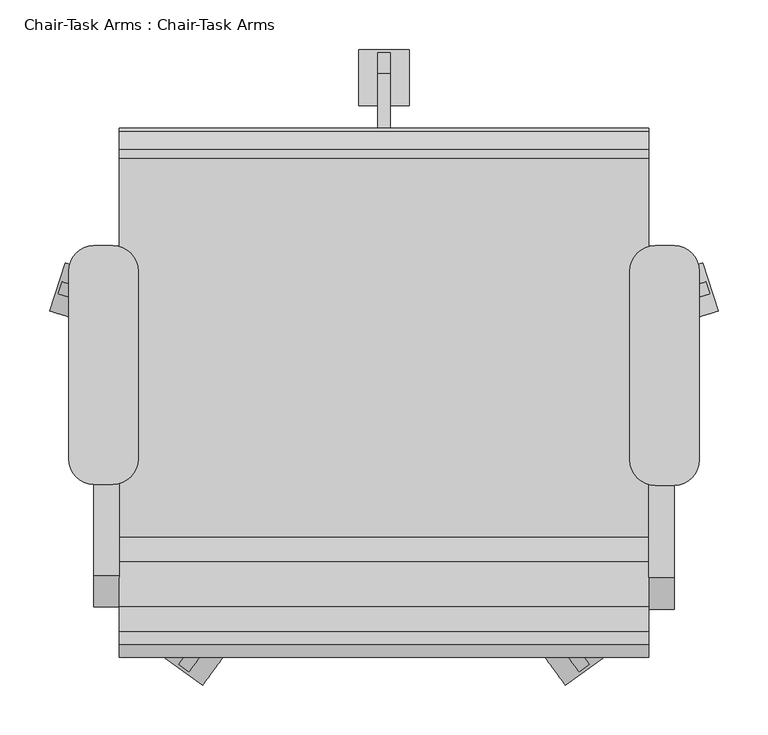
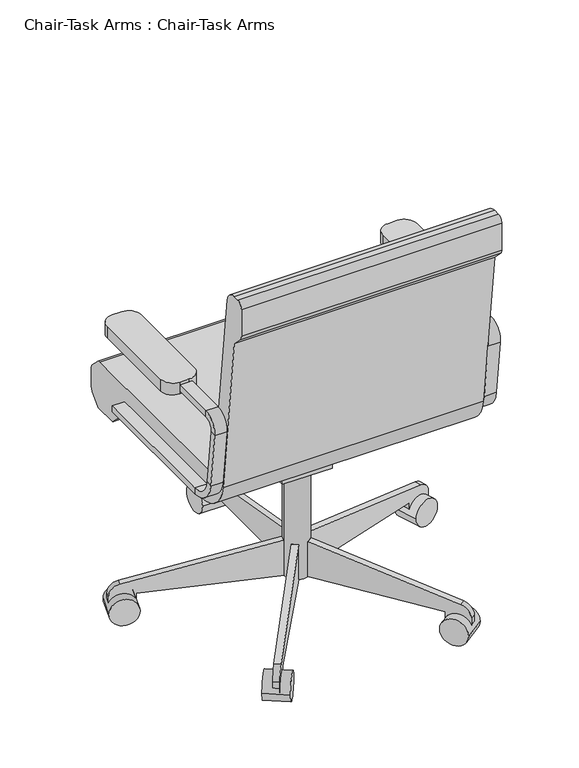
"""IFC4 building model written with IfcOpenShell, lengths in millimetres: furniture geometry, Chair-Task Arms : Chair-Task Arms."""

from ifc_helpers import new_model, si_unit, point, frame, frame_2d, origin, place, context, project, spatial, polyline, circle_curve, trimmed, segment, composite_curve, outline, extrude, source, transform, mapped, element, save
from ifc_brep_helpers import plane_surface, cylinder_surface, revolved_surface, advanced_brep


def chair_task_arms_chair_task_arms_bb362225(model_context):
    return source(origin(), model_context, "Body", "SolidModel", [
        extrude(outline(composite_curve([segment(polyline([(-126.2050455, 457.2), (255.0102301, 457.2)]), True, "CONTINUOUS"), segment(trimmed(circle_curve(frame_2d((255.0102301, 444.5)), 12.7), [point((255.0102301, 457.2))], [point((263.9604301, 453.510212))], False, "CARTESIAN"), True, "CONTINUOUS"), segment(polyline([(263.9604301, 453.510212), (281.8961016, 435.6939999)]), True, "CONTINUOUS"), segment(trimmed(circle_curve(frame_2d((272.9459016, 426.6837879)), 12.7), [point((281.8961016, 435.6939999))], [point((285.6459016, 426.6837879))], False, "CARTESIAN"), True, "CONTINUOUS"), segment(polyline([(285.6459016, 426.6837879), (285.6459016, 391.6405184)]), True, "CONTINUOUS"), segment(trimmed(circle_curve(frame_2d((260.2459016, 391.6405184)), 25.4), [point((285.6459016, 391.6405184))], [point((278.2663256, 373.7401184))], False, "CARTESIAN"), True, "CONTINUOUS"), segment(polyline([(278.2663256, 373.7401184), (260.2470284, 355.6), (209.4470284, 355.6), (181.0744602, 383.7835944), (-107.1089978, 383.7835944)]), True, "CONTINUOUS"), segment(trimmed(circle_curve(frame_2d((-107.1089978, 459.9835944)), 76.2), [point((-107.1089978, 383.7835944))], [point((-182.7870738, 451.0802913))], False, "CARTESIAN"), True, "CONTINUOUS"), segment(polyline([(-182.7870738, 451.0802913), (-222.3540984, 787.4), (-244.0343545, 809.0802561)]), True, "CONTINUOUS"), segment(trimmed(circle_curve(frame_2d((-235.0540984, 818.0605122)), 12.7), [point((-244.0343545, 809.0802561))], [point((-247.7540984, 818.0605122))], False, "CARTESIAN"), True, "CONTINUOUS"), segment(polyline([(-247.7540984, 818.0605122), (-247.7540984, 876.3)]), True, "CONTINUOUS"), segment(trimmed(circle_curve(frame_2d((-235.0540984, 876.3)), 12.7), [point((-247.7540984, 876.3))], [point((-235.0540984, 889.0))], False, "CARTESIAN"), True, "CONTINUOUS"), segment(polyline([(-235.0540984, 889.0), (-222.1789239, 889.0)]), True, "CONTINUOUS"), segment(trimmed(circle_curve(frame_2d((-222.1789239, 863.6)), 25.4), [point((-222.1789239, 889.0))], [point((-196.9528985, 866.5677677))], False, "CARTESIAN"), True, "CONTINUOUS"), segment(polyline([(-196.9528985, 866.5677677), (-151.4310708, 479.6322323)]), True, "CONTINUOUS"), segment(trimmed(circle_curve(frame_2d((-126.2050455, 482.6)), 25.4), [point((-151.4310708, 479.6322323))], [point((-126.2050455, 457.2))], True, "CARTESIAN"), True, "CONTINUOUS")], self_intersect=False)), frame((-125.7091803, 0.0, 0.0), z_axis=(1.0, 0.0, 0.0), x_axis=(0.0, 1.0, 0.0)), (0.0, 0.0, 1.0), 533.4),
        extrude(outline(polyline([(69.7459016, 383.7835944), (69.7459016, 371.0835944), (18.9459016, 283.0954134), (-19.1540984, 283.0954134), (-19.1540984, 383.7835944), (69.7459016, 383.7835944)])), frame((90.1908197, 0.0, 0.0), z_axis=(1.0, 0.0, 0.0), x_axis=(0.0, 1.0, 0.0)), (0.0, 0.0, 1.0), 101.6),
        extrude(outline(composite_curve([segment(polyline([(311.0459016, 53.5835944), (18.9459016, 53.5835944), (18.9459016, 129.7835944), (44.3459016, 129.7835944), (340.8565654, 77.5007643)]), True, "CONTINUOUS"), segment(trimmed(circle_curve(frame_2d((336.4459016, 52.4866474)), 25.4), [point((340.8565654, 77.5007643))], [point((361.8459016, 52.4866474))], False, "CARTESIAN"), True, "CONTINUOUS"), segment(polyline([(361.8459016, 52.4866474), (361.8459016, 28.1835944), (311.0459016, 28.1835944), (311.0459016, 53.5835944)]), True, "CONTINUOUS")], self_intersect=False)), frame((134.6408197, 0.0, 0.0), z_axis=(1.0, 0.0, 0.0), x_axis=(0.0, 1.0, 0.0)), (0.0, 0.0, 1.0), 12.7),
        extrude(outline(composite_curve([segment(trimmed(circle_curve(frame_2d((336.4459016, 28.1835944)), 28.2002727), [point((308.2456289, 28.1835944))], [point((364.6461744, 28.1835944))], False, "CARTESIAN"), True, "CONTINUOUS"), segment(trimmed(circle_curve(frame_2d((336.4459016, 28.1835944)), 28.2002727), [point((364.6461744, 28.1835944))], [point((308.2456289, 28.1835944))], False, "CARTESIAN"), True, "CONTINUOUS")], self_intersect=False)), frame((115.5908197, 0.0, 0.0), z_axis=(1.0, 0.0, 0.0), x_axis=(0.0, 1.0, 0.0)), (0.0, 0.0, 1.0), 50.8),
        extrude(outline(composite_curve([segment(polyline([(25.4, 0.0), (25.4, 292.1000001), (101.6, 292.1000001), (101.6, 266.7), (49.3171699, -29.8106636)]), True, "CONTINUOUS"), segment(trimmed(circle_curve(frame_2d((24.303053, -25.4)), 25.4), [point((49.3171699, -29.8106636))], [point((24.303053, -50.8))], False, "CARTESIAN"), True, "CONTINUOUS"), segment(polyline([(24.303053, -50.8), (0.0, -50.8), (0.0, 0.0), (25.4, 0.0)]), True, "CONTINUOUS")], self_intersect=False)), frame((-138.7750467, 103.1705568, 28.1835944), z_axis=(0.3090169943749487, 0.9510565162951532, 0.0), x_axis=(0.0, 0.0, 1.0)), (0.0, 0.0, 1.0), 12.7),
        extrude(outline(composite_curve([segment(trimmed(circle_curve(frame_2d((0.0, -28.2002727)), 28.2002727), [point((0.0, -56.4005454))], [point((0.0, 0.0))], False, "CARTESIAN"), True, "CONTINUOUS"), segment(trimmed(circle_curve(frame_2d((0.0, -28.2002727)), 28.2002727), [point((0.0, 0.0))], [point((0.0, -56.4005454))], False, "CARTESIAN"), True, "CONTINUOUS")], self_intersect=False)), frame((-195.638709, 101.6163254, 28.1835944), z_axis=(0.3090169943749487, 0.9510565162951532, 0.0), x_axis=(0.0, 0.0, -1.0)), (0.0, 0.0, 1.0), 50.8),
        extrude(outline(composite_curve([segment(polyline([(25.4, 0.0), (25.4, 292.1), (101.6, 292.1), (101.6, 266.7), (49.3171699, -29.8106637)]), True, "CONTINUOUS"), segment(trimmed(circle_curve(frame_2d((24.303053, -25.3999999)), 25.4), [point((49.3171699, -29.8106637))], [point((24.303053, -50.8))], False, "CARTESIAN"), True, "CONTINUOUS"), segment(polyline([(24.303053, -50.8), (0.0, -50.8), (0.0, 0.0), (25.4, 0.0)]), True, "CONTINUOUS")], self_intersect=False)), frame((-25.5639946, -221.1003988, 28.1835944), z_axis=(-0.8090169943749459, 0.5877852522924754, 0.0), x_axis=(0.0, 0.0, 1.0)), (0.0, 0.0, 1.0), 12.7),
        extrude(outline(composite_curve([segment(trimmed(circle_curve(frame_2d((0.0, -28.2002727)), 28.2002727), [point((0.0, -56.4005455))], [point((0.0, 0.0))], False, "CARTESIAN"), True, "CONTINUOUS"), segment(trimmed(circle_curve(frame_2d((0.0, -28.2002727)), 28.2002727), [point((0.0, 0.0))], [point((0.0, -56.4005455))], False, "CARTESIAN"), True, "CONTINUOUS")], self_intersect=False)), frame((-41.6576707, -275.6612394, 28.1835944), z_axis=(-0.8090169943749458, 0.5877852522924754, 0.0), x_axis=(0.0, 0.0, -1.0)), (0.0, 0.0, 1.0), 50.8),
        extrude(outline(composite_curve([segment(polyline([(-25.4, 0.0), (0.0, 0.0), (0.0, -50.8), (-24.303053, -50.8)]), True, "CONTINUOUS"), segment(trimmed(circle_curve(frame_2d((-24.303053, -25.3999999)), 25.4), [point((-24.303053, -50.8))], [point((-49.3171699, -29.8106636))], False, "CARTESIAN"), True, "CONTINUOUS"), segment(polyline([(-49.3171699, -29.8106636), (-101.6, 266.7), (-101.6, 292.1), (-25.4, 292.1), (-25.4, 0.0)]), True, "CONTINUOUS")], self_intersect=False)), frame((307.545634, -221.1003988, 28.1835944), z_axis=(0.8090169943749499, 0.5877852522924699, 0.0), x_axis=(0.0, 0.0, -1.0)), (0.0, 0.0, 1.0), 12.7),
        extrude(outline(composite_curve([segment(trimmed(circle_curve(frame_2d((0.0, -28.2002727)), 28.2002727), [point((0.0, -56.4005455))], [point((0.0, 0.0))], False, "CARTESIAN"), True, "CONTINUOUS"), segment(trimmed(circle_curve(frame_2d((0.0, -28.2002727)), 28.2002727), [point((0.0, 0.0))], [point((0.0, -56.4005455))], False, "CARTESIAN"), True, "CONTINUOUS")], self_intersect=False)), frame((323.63931, -275.6612394, 28.1835944), z_axis=(0.8090169943749499, 0.5877852522924699, 0.0), x_axis=(0.0, 0.0, 1.0)), (0.0, 0.0, 1.0), 50.8),
        extrude(outline(composite_curve([segment(polyline([(-25.4, 0.0), (0.0, 0.0), (0.0, -50.8), (-24.303053, -50.8)]), True, "CONTINUOUS"), segment(trimmed(circle_curve(frame_2d((-24.303053, -25.4)), 25.4), [point((-24.303053, -50.8))], [point((-49.3171699, -29.8106637))], False, "CARTESIAN"), True, "CONTINUOUS"), segment(polyline([(-49.3171699, -29.8106637), (-101.6, 266.7), (-101.6, 292.1), (-25.4, 292.1), (-25.4, 0.0)]), True, "CONTINUOUS")], self_intersect=False)), frame((420.756686, 103.1705568, 28.1835944), z_axis=(-0.3090169943749423, 0.9510565162951553, 0.0), x_axis=(0.0, 0.0, -1.0)), (0.0, 0.0, 1.0), 12.7),
        extrude(outline(composite_curve([segment(trimmed(circle_curve(frame_2d((0.0, -28.2002727)), 28.2002727), [point((0.0, -56.4005455))], [point((0.0, 0.0))], False, "CARTESIAN"), True, "CONTINUOUS"), segment(trimmed(circle_curve(frame_2d((0.0, -28.2002727)), 28.2002727), [point((0.0, 0.0))], [point((0.0, -56.4005455))], False, "CARTESIAN"), True, "CONTINUOUS")], self_intersect=False)), frame((477.6203484, 101.6163254, 28.1835944), z_axis=(-0.3090169943749423, 0.9510565162951553, 0.0), x_axis=(0.0, 0.0, 1.0)), (0.0, 0.0, 1.0), 50.8),
        extrude(outline(composite_curve([segment(trimmed(circle_curve(frame_2d((140.9908197, 18.9459016)), 25.4), [point((115.5908197, 18.9459016))], [point((166.3908197, 18.9459016))], False, "CARTESIAN"), True, "CONTINUOUS"), segment(trimmed(circle_curve(frame_2d((140.9908197, 18.9459016)), 25.4), [point((166.3908197, 18.9459016))], [point((115.5908197, 18.9459016))], False, "CARTESIAN"), True, "CONTINUOUS")], self_intersect=False)), frame((0.0, 0.0, 53.5835944), z_axis=(0.0, 0.0, 1.0), x_axis=(1.0, 0.0, 0.0)), (0.0, 0.0, 1.0), 330.5914056),
        advanced_brep(
        [(433.0908197, 167.0319091, 425.45), (433.0908197, 167.0319091, 412.75), (407.6908197, 167.0319091, 412.75), (407.6908197, 167.0319091, 425.45), (433.0908197, -128.329278, 425.45), (433.0908197, -128.329278, 412.75), (407.6908197, -128.329278, 412.75), (407.6908197, -128.329278, 425.45), (433.0908197, -185.0878351, 463.2225227), (433.0908197, -172.4748224, 464.7064065), (407.6908197, -185.0878351, 463.2225227), (407.6908197, -172.4748224, 464.7064065), (433.0908197, -186.2710303, 581.9741742), (433.0908197, -198.884043, 580.4902904), (407.6908197, -198.884043, 580.4902904), (407.6908197, -186.2710303, 581.9741742), (433.0908197, -167.3515113, 615.95), (433.0908197, -167.3515113, 603.25), (407.6908197, -167.3515113, 615.95), (407.6908197, -167.3515113, 603.25), (433.0908197, 18.9459016, 603.25), (407.6908197, 18.9459016, 603.25), (407.6908197, 18.9459016, 615.95), (433.0908197, 18.9459016, 615.95)],
        [
            (0, 1),
            (1, 2),
            (2, 3),
            (3, 0),
            (0, 4),
            (4, 5),
            (5, 1),
            (5, 6),
            (6, 2),
            (6, 7),
            (7, 3),
            (7, 4),
            (8, 5, circle_curve(frame((433.0908197, -128.329278, 469.9), z_axis=(1.0, 0.0, 0.0), x_axis=(0.0, 0.0, -1.0)), 57.15)),
            (4, 9, circle_curve(frame((433.0908197, -128.329278, 469.9), z_axis=(-1.0, 0.0, 0.0), x_axis=(0.0, 0.0, -1.0)), 44.45)),
            (9, 8),
            (10, 6, circle_curve(frame((407.6908197, -128.329278, 469.9), z_axis=(1.0, 0.0, 0.0), x_axis=(0.0, 0.0, -1.0)), 57.15)),
            (8, 10),
            (11, 7, circle_curve(frame((407.6908197, -128.329278, 469.9), z_axis=(1.0, 0.0, 0.0), x_axis=(0.0, 0.0, -1.0)), 44.45)),
            (10, 11),
            (11, 9),
            (9, 12),
            (12, 13),
            (13, 8),
            (13, 14),
            (14, 10),
            (14, 15),
            (15, 11),
            (15, 12),
            (16, 13, circle_curve(frame((433.0908197, -167.3515113, 584.2), z_axis=(1.0, 0.0, 0.0), x_axis=(0.0, -0.9931506043228767, -0.1168412475673929)), 31.75)),
            (12, 17, circle_curve(frame((433.0908197, -167.3515113, 584.2), z_axis=(-1.0, 0.0, 0.0), x_axis=(0.0, -0.9931506043228767, -0.1168412475673929)), 19.05)),
            (17, 16),
            (18, 14, circle_curve(frame((407.6908197, -167.3515113, 584.2), z_axis=(1.0, 0.0, 0.0), x_axis=(0.0, -0.9931506043228767, -0.1168412475673929)), 31.75)),
            (16, 18),
            (19, 15, circle_curve(frame((407.6908197, -167.3515113, 584.2), z_axis=(1.0, 0.0, 0.0), x_axis=(0.0, -0.9931506043228767, -0.1168412475673929)), 19.05)),
            (18, 19),
            (19, 17),
            (20, 21),
            (21, 22),
            (22, 23),
            (23, 20),
            (17, 20),
            (23, 16),
            (22, 18),
            (21, 19),
        ],
        [
            plane_surface(frame((406.191788, 167.0319091, 419.1), z_axis=(0.0, 1.0, 0.0), x_axis=(0.0, 0.0, -1.0))),
            plane_surface(frame((433.0908197, 167.0319091, 425.45), z_axis=(1.0, 0.0, 0.0), x_axis=(0.0, -1.0, 0.0))),
            plane_surface(frame((433.0908197, 167.0319091, 412.75), z_axis=(0.0, 0.0, -1.0), x_axis=(0.0, -1.0, 0.0))),
            plane_surface(frame((407.6908197, 167.0319091, 412.75), z_axis=(-1.0, 0.0, 0.0), x_axis=(0.0, -1.0, 0.0))),
            plane_surface(frame((407.6908197, 167.0319091, 425.45), z_axis=(0.0, 0.0, 1.0), x_axis=(0.0, -1.0, 0.0))),
            plane_surface(frame((433.0908197, -128.329278, 469.9), z_axis=(1.0, 0.0, 0.0), x_axis=(0.0, 0.0, -1.0))),
            cylinder_surface(frame((420.3908197, -128.329278, 469.9), z_axis=(-1.0, 0.0, 0.0), x_axis=(0.0, 0.0, -1.0)), 57.15),
            plane_surface(frame((407.6908197, -128.329278, 469.9), z_axis=(-1.0, 0.0, 0.0), x_axis=(0.0, 0.0, -1.0))),
            revolved_surface(polyline([(407.6908197, -128.329278, 425.45), (433.0908197, -128.329278, 425.45)]), (420.3908197, -128.329278, 469.9), (-1.0, 0.0, 0.0)),
            plane_surface(frame((433.0908197, -172.4748224, 464.7064065), z_axis=(1.0, 0.0, 0.0), x_axis=(0.0, -0.11684124756738626, 0.9931506043228775))),
            plane_surface(frame((433.0908197, -185.0878351, 463.2225227), z_axis=(0.0, -0.9931506043228775, -0.11684124756738655), x_axis=(0.0, -0.11684124756738655, 0.9931506043228775))),
            plane_surface(frame((407.6908197, -185.0878351, 463.2225227), z_axis=(-1.0, 0.0, 0.0), x_axis=(0.0, -0.11684124756738626, 0.9931506043228775))),
            plane_surface(frame((407.6908197, -172.4748224, 464.7064065), z_axis=(0.0, 0.9931506043228775, 0.11684124756738626), x_axis=(0.0, -0.11684124756738626, 0.9931506043228775))),
            plane_surface(frame((433.0908197, -167.3515113, 584.2), z_axis=(1.0, 0.0, 0.0), x_axis=(0.0, -0.9931506043228767, -0.1168412475673929))),
            cylinder_surface(frame((420.3908197, -167.3515113, 584.2), z_axis=(-1.0, 0.0, 0.0), x_axis=(0.0, -0.9931506043228767, -0.1168412475673929)), 31.75),
            plane_surface(frame((407.6908197, -167.3515113, 584.2), z_axis=(-1.0, 0.0, 0.0), x_axis=(0.0, -0.9931506043228767, -0.1168412475673929))),
            revolved_surface(polyline([(407.6908197, -186.2710303123508, 581.9741742338412), (433.0908197, -186.2710303123508, 581.9741742338412)]), (420.3908197, -167.3515113, 584.2), (-1.0, 0.0, 0.0)),
            plane_surface(frame((406.191788, 18.9459016, 609.6), z_axis=(0.0, 1.0, 0.0), x_axis=(0.0, 0.0, 1.0))),
            plane_surface(frame((433.0908197, -167.3515113, 603.25), z_axis=(1.0, 0.0, 0.0), x_axis=(0.0, 1.0, 0.0))),
            plane_surface(frame((433.0908197, -167.3515113, 615.95), z_axis=(0.0, 0.0, 1.0), x_axis=(0.0, 1.0, 0.0))),
            plane_surface(frame((407.6908197, -167.3515113, 615.95), z_axis=(-1.0, 0.0, 0.0), x_axis=(0.0, 1.0, 0.0))),
            plane_surface(frame((407.6908197, -167.3515113, 603.25), z_axis=(0.0, 0.0, -1.0), x_axis=(0.0, 1.0, 0.0))),
        ],
        [
            (0, [[1, 2, 3, 4]]),
            (1, [[-1, 5, 6, 7]]),
            (2, [[-2, -7, 8, 9]]),
            (3, [[-3, -9, 10, 11]]),
            (4, [[-4, -11, 12, -5]]),
            (5, [[13, -6, 14, 15]]),
            (6, [[16, -8, -13, 17]]),
            (7, [[18, -10, -16, 19]]),
            (8, [[-14, -12, -18, 20]]),
            (9, [[-15, 21, 22, 23]]),
            (10, [[-17, -23, 24, 25]]),
            (11, [[-19, -25, 26, 27]]),
            (12, [[-20, -27, 28, -21]]),
            (13, [[29, -22, 30, 31]]),
            (14, [[32, -24, -29, 33]]),
            (15, [[34, -26, -32, 35]]),
            (16, [[-30, -28, -34, 36]]),
            (17, [[37, 38, 39, 40]]),
            (18, [[-31, 41, -40, 42]]),
            (19, [[-33, -42, -39, 43]]),
            (20, [[-35, -43, -38, 44]]),
            (21, [[-36, -44, -37, -41]]),
        ],
    ),
        advanced_brep(
        [(-151.1091803, 167.0319091, 412.75), (-151.1091803, 167.0319091, 425.45), (-125.7091803, 167.0319091, 425.45), (-125.7091803, 167.0319091, 412.75), (-151.1091803, -126.2388651, 412.75), (-151.1091803, -126.2388651, 425.45), (-125.7091803, -126.2388651, 425.45), (-125.7091803, -126.2388651, 412.75), (-151.1091803, -170.3844094, 464.7064065), (-151.1091803, -182.9974221, 463.2225227), (-125.7091803, -170.3844094, 464.7064065), (-125.7091803, -182.9974221, 463.2225227), (-151.1091803, -196.7936301, 580.4902904), (-151.1091803, -184.1806174, 581.9741742), (-125.7091803, -184.1806174, 581.9741742), (-125.7091803, -196.7936301, 580.4902904), (-151.1091803, -165.2610984, 603.25), (-151.1091803, -165.2610984, 615.95), (-125.7091803, -165.2610984, 603.25), (-125.7091803, -165.2610984, 615.95), (-151.1091803, 18.9459016, 615.95), (-125.7091803, 18.9459016, 615.95), (-125.7091803, 18.9459016, 603.25), (-151.1091803, 18.9459016, 603.25)],
        [
            (0, 1),
            (1, 2),
            (2, 3),
            (3, 0),
            (0, 4),
            (4, 5),
            (5, 1),
            (5, 6),
            (6, 2),
            (6, 7),
            (7, 3),
            (7, 4),
            (8, 5, circle_curve(frame((-151.1091803, -126.2388651, 469.9), z_axis=(1.0, 0.0, 0.0), x_axis=(0.0, 0.0, -1.0)), 44.45)),
            (4, 9, circle_curve(frame((-151.1091803, -126.2388651, 469.9), z_axis=(-1.0, 0.0, 0.0), x_axis=(0.0, 0.0, -1.0)), 57.15)),
            (9, 8),
            (10, 6, circle_curve(frame((-125.7091803, -126.2388651, 469.9), z_axis=(1.0, 0.0, 0.0), x_axis=(0.0, 0.0, -1.0)), 44.45)),
            (8, 10),
            (11, 7, circle_curve(frame((-125.7091803, -126.2388651, 469.9), z_axis=(1.0, 0.0, 0.0), x_axis=(0.0, 0.0, -1.0)), 57.15)),
            (10, 11),
            (11, 9),
            (9, 12),
            (12, 13),
            (13, 8),
            (13, 14),
            (14, 10),
            (14, 15),
            (15, 11),
            (15, 12),
            (16, 13, circle_curve(frame((-151.1091803, -165.2610984, 584.2), z_axis=(1.0, 0.0, 0.0), x_axis=(0.0, -0.9931506043228768, -0.11684124756739202)), 19.05)),
            (12, 17, circle_curve(frame((-151.1091803, -165.2610984, 584.2), z_axis=(-1.0, 0.0, 0.0), x_axis=(0.0, -0.9931506043228768, -0.11684124756739202)), 31.75)),
            (17, 16),
            (18, 14, circle_curve(frame((-125.7091803, -165.2610984, 584.2), z_axis=(1.0, 0.0, 0.0), x_axis=(0.0, -0.9931506043228768, -0.11684124756739202)), 19.05)),
            (16, 18),
            (19, 15, circle_curve(frame((-125.7091803, -165.2610984, 584.2), z_axis=(1.0, 0.0, 0.0), x_axis=(0.0, -0.9931506043228768, -0.11684124756739202)), 31.75)),
            (18, 19),
            (19, 17),
            (20, 21),
            (21, 22),
            (22, 23),
            (23, 20),
            (17, 20),
            (23, 16),
            (22, 18),
            (21, 19),
        ],
        [
            plane_surface(frame((-152.608212, 167.0319091, 419.1), z_axis=(0.0, 1.0, 0.0), x_axis=(0.0, 0.0, -1.0))),
            plane_surface(frame((-151.1091803, 167.0319091, 412.75), z_axis=(-1.0, 0.0, 0.0), x_axis=(0.0, -1.0, 0.0))),
            plane_surface(frame((-151.1091803, 167.0319091, 425.45), z_axis=(0.0, 0.0, 1.0), x_axis=(0.0, -1.0, 0.0))),
            plane_surface(frame((-125.7091803, 167.0319091, 425.45), z_axis=(1.0, 0.0, 0.0), x_axis=(0.0, -1.0, 0.0))),
            plane_surface(frame((-125.7091803, 167.0319091, 412.75), z_axis=(0.0, 0.0, -1.0), x_axis=(0.0, -1.0, 0.0))),
            plane_surface(frame((-151.1091803, -126.2388651, 469.9), z_axis=(-1.0, 0.0, 0.0), x_axis=(0.0, 0.0, -1.0))),
            revolved_surface(polyline([(-151.1091803, -126.2388651, 425.45), (-125.7091803, -126.2388651, 425.45)]), (-138.4091803, -126.2388651, 469.9), (-1.0, 0.0, 0.0)),
            plane_surface(frame((-125.7091803, -126.2388651, 469.9), z_axis=(1.0, 0.0, 0.0), x_axis=(0.0, 0.0, -1.0))),
            cylinder_surface(frame((-138.4091803, -126.2388651, 469.9), z_axis=(-1.0, 0.0, 0.0), x_axis=(0.0, 0.0, -1.0)), 57.15),
            plane_surface(frame((-151.1091803, -182.9974221, 463.2225227), z_axis=(-1.0, 0.0, 0.0), x_axis=(0.0, -0.1168412475673856, 0.9931506043228776))),
            plane_surface(frame((-151.1091803, -170.3844094, 464.7064065), z_axis=(0.0, 0.9931506043228776, 0.1168412475673856), x_axis=(0.0, -0.1168412475673856, 0.9931506043228776))),
            plane_surface(frame((-125.7091803, -170.3844094, 464.7064065), z_axis=(1.0, 0.0, 0.0), x_axis=(0.0, -0.1168412475673856, 0.9931506043228776))),
            plane_surface(frame((-125.7091803, -182.9974221, 463.2225227), z_axis=(0.0, -0.9931506043228776, -0.1168412475673856), x_axis=(0.0, -0.1168412475673856, 0.9931506043228776))),
            plane_surface(frame((-151.1091803, -165.2610984, 584.2), z_axis=(-1.0, 0.0, 0.0), x_axis=(0.0, -0.9931506043228768, -0.11684124756739202))),
            revolved_surface(polyline([(-151.1091803, -184.1806174123508, 581.9741742338413), (-125.7091803, -184.1806174123508, 581.9741742338413)]), (-138.4091803, -165.2610984, 584.2), (-1.0, 0.0, 0.0)),
            plane_surface(frame((-125.7091803, -165.2610984, 584.2), z_axis=(1.0, 0.0, 0.0), x_axis=(0.0, -0.9931506043228768, -0.11684124756739202))),
            cylinder_surface(frame((-138.4091803, -165.2610984, 584.2), z_axis=(-1.0, 0.0, 0.0), x_axis=(0.0, -0.9931506043228768, -0.11684124756739202)), 31.75),
            plane_surface(frame((-152.608212, 18.9459016, 609.6), z_axis=(0.0, 1.0, 0.0), x_axis=(0.0, 0.0, 1.0))),
            plane_surface(frame((-151.1091803, -165.2610984, 615.95), z_axis=(-1.0, 0.0, 0.0), x_axis=(0.0, 1.0, 0.0))),
            plane_surface(frame((-151.1091803, -165.2610984, 603.25), z_axis=(0.0, 0.0, -1.0), x_axis=(0.0, 1.0, 0.0))),
            plane_surface(frame((-125.7091803, -165.2610984, 603.25), z_axis=(1.0, 0.0, 0.0), x_axis=(0.0, 1.0, 0.0))),
            plane_surface(frame((-125.7091803, -165.2610984, 615.95), z_axis=(0.0, 0.0, 1.0), x_axis=(0.0, 1.0, 0.0))),
        ],
        [
            (0, [[1, 2, 3, 4]]),
            (1, [[-1, 5, 6, 7]]),
            (2, [[-2, -7, 8, 9]]),
            (3, [[-3, -9, 10, 11]]),
            (4, [[-4, -11, 12, -5]]),
            (5, [[13, -6, 14, 15]]),
            (6, [[16, -8, -13, 17]]),
            (7, [[18, -10, -16, 19]]),
            (8, [[-14, -12, -18, 20]]),
            (9, [[-15, 21, 22, 23]]),
            (10, [[-17, -23, 24, 25]]),
            (11, [[-19, -25, 26, 27]]),
            (12, [[-20, -27, 28, -21]]),
            (13, [[29, -22, 30, 31]]),
            (14, [[32, -24, -29, 33]]),
            (15, [[34, -26, -32, 35]]),
            (16, [[-30, -28, -34, 36]]),
            (17, [[37, 38, 39, 40]]),
            (18, [[-31, 41, -40, 42]]),
            (19, [[-33, -42, -39, 43]]),
            (20, [[-35, -43, -38, 44]]),
            (21, [[-36, -44, -37, -41]]),
        ],
    ),
        extrude(outline(composite_curve([segment(polyline([(433.0908197, -74.2028048), (414.0408197, -74.2028048)]), True, "CONTINUOUS"), segment(trimmed(circle_curve(frame_2d((414.0408197, -48.8028048)), 25.4), [point((414.0408197, -74.2028048))], [point((388.6408197, -48.8028048))], False, "CARTESIAN"), True, "CONTINUOUS"), segment(polyline([(388.6408197, -48.8028048), (388.6408197, 141.6319091)]), True, "CONTINUOUS"), segment(trimmed(circle_curve(frame_2d((414.0408197, 141.6319091)), 25.4), [point((388.6408197, 141.6319091))], [point((414.0408197, 167.0319091))], False, "CARTESIAN"), True, "CONTINUOUS"), segment(polyline([(414.0408197, 167.0319091), (433.0908197, 167.0319091)]), True, "CONTINUOUS"), segment(trimmed(circle_curve(frame_2d((433.0908197, 141.6319091)), 25.4), [point((433.0908197, 167.0319091))], [point((458.4908197, 141.6319091))], False, "CARTESIAN"), True, "CONTINUOUS"), segment(polyline([(458.4908197, 141.6319091), (458.4908197, -48.8028048)]), True, "CONTINUOUS"), segment(trimmed(circle_curve(frame_2d((433.0908197, -48.8028048)), 25.4), [point((458.4908197, -48.8028048))], [point((433.0908197, -74.2028048))], False, "CARTESIAN"), True, "CONTINUOUS")], self_intersect=False)), frame((0.0, 0.0, 596.9), z_axis=(0.0, 0.0, 1.0), x_axis=(1.0, 0.0, 0.0)), (0.0, 0.0, 1.0), 25.4),
        extrude(outline(composite_curve([segment(polyline([(-132.0591803, -73.1575984), (-151.1091803, -73.1575984)]), True, "CONTINUOUS"), segment(trimmed(circle_curve(frame_2d((-151.1091803, -47.7575984)), 25.4), [point((-151.1091803, -73.1575984))], [point((-176.5091803, -47.7575984))], False, "CARTESIAN"), True, "CONTINUOUS"), segment(polyline([(-176.5091803, -47.7575984), (-176.5091803, 141.6319091)]), True, "CONTINUOUS"), segment(trimmed(circle_curve(frame_2d((-151.1091803, 141.6319091)), 25.4), [point((-176.5091803, 141.6319091))], [point((-151.1091803, 167.0319091))], False, "CARTESIAN"), True, "CONTINUOUS"), segment(polyline([(-151.1091803, 167.0319091), (-132.0591803, 167.0319091)]), True, "CONTINUOUS"), segment(trimmed(circle_curve(frame_2d((-132.0591803, 141.6319091)), 25.4), [point((-132.0591803, 167.0319091))], [point((-106.6591803, 141.6319091))], False, "CARTESIAN"), True, "CONTINUOUS"), segment(polyline([(-106.6591803, 141.6319091), (-106.6591803, -47.7575984)]), True, "CONTINUOUS"), segment(trimmed(circle_curve(frame_2d((-132.0591803, -47.7575984)), 25.4), [point((-106.6591803, -47.7575984))], [point((-132.0591803, -73.1575984))], False, "CARTESIAN"), True, "CONTINUOUS")], self_intersect=False)), frame((0.0, 0.0, 596.9), z_axis=(0.0, 0.0, 1.0), x_axis=(1.0, 0.0, 0.0)), (0.0, 0.0, 1.0), 25.4),
    ])


if __name__ == "__main__":
    model = new_model("IFC4")
    model_context = context("Model", 3, world=origin())
    ifc_project = project(units=[si_unit("LENGTHUNIT", "METRE", prefix="MILLI")], contexts=[model_context])
    site = spatial("IfcSite", under=ifc_project)
    building = spatial("IfcBuilding", under=site)
    placement = place(None, origin())
    chair_task_arms_chair_task_arms_shape = chair_task_arms_chair_task_arms_bb362225(model_context)
    element("IfcFurniture", 1, ObjectType="Chair-Task Arms : Chair-Task Arms", at=placement, inside=building, context=model_context, shape_type="MappedRepresentation", body=[
        mapped(chair_task_arms_chair_task_arms_shape, transform((0.0, 0.0, 0.0), x_axis=(1.0, 0.0, 0.0), y_axis=(0.0, 1.0, 0.0), z_axis=(0.0, 0.0, 1.0))),
    ])
    save(model, "model.ifc")

# Revit data of these elements
# Type "Chair-Task Arms : Chair-Task Arms"
#   Assembly Code = "E2020200"
#   Base Material = Plastic, Opaque Black
#   Caster Material = Plastic, Opaque Black
#   Seat/Back Material = Textile - Slate Blue
#   Default Elevation = 0
# Element 1 (IfcFurniture, "Chair-Task Arms : Chair-Task Arms")
#   Materials on its faces: "Plastic, Opaque Black", "Textile - Slate Blue"
# Materials
#   "Plastic, Opaque Black": class "Plastic", colour RGB 0 0 0, transparency 0, Description = "Plastic, generic, opaque black", Cost = 0
#   "Textile - Slate Blue": class "Fabric", colour RGB 98 102 118, transparency 0
